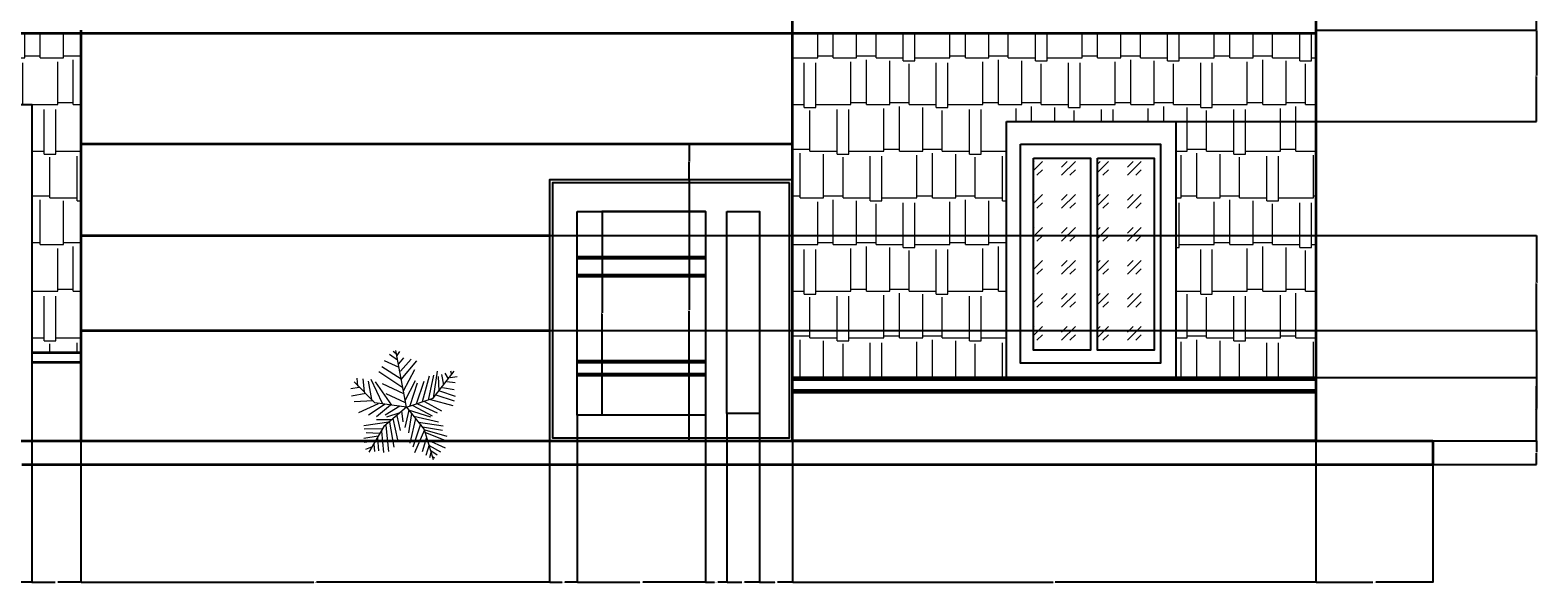
# Model space of a CAD drawing. Units: inches. Extents: x -73 to 2199, y -12 to 1583.
# Tile 2 of 3: x 686 to 2199, y -12 to 543. Entities that reach past the tile are written whole.
import ezdxf

# ---------------------------------------------------------------- set-up
doc = ezdxf.new("R2010")
doc.units = ezdxf.units.IN
doc.header["$MEASUREMENT"] = 0
for name, color, linetype, lineweight in [('A-ANNO-DIMS', 2, 'Continuous', 18), ('A-DOOR', 3, 'Continuous', 25), ('A-ELEV', 7, 'Continuous', 35), ('A-GLAZ', 4, 'Continuous', 25), ('A-GLAZ-PATT', 8, 'Continuous', 13), ('A-WALL-PATT', 8, 'Continuous', 13), ('L-PLNT', 3, 'Continuous', 18)]:
    doc.layers.add(name, color=color, linetype=linetype, lineweight=lineweight)
doc.styles.get("Standard").update_dxf_attribs({"font": 'arial.ttf'})
doc.dimstyles.get("Standard").update_dxf_attribs({"dimtxt": 0.75, "dimasz": 0.18, "dimexe": 0.18, "dimexo": 0.0625, "dimgap": 0.09, "dimtad": 0, "dimtih": 1, "dimtoh": 1, "dimdec": 4, "dimzin": 0, "dimdsep": 46, "dimlunit": 4, "dimtxsty": 'Standard', "dimcen": 0.09, "dimadec": 0, "dimazin": 0, "dimtfac": 1, "dimtdec": 4, "dimtofl": 0, "dimtmove": 0, "dimatfit": 3, "dimfxl": 1, "dimtolj": 1, "dimtzin": 0, "dimarcsym": 0})

# ---------------------------------------------------------------- blocks, each defined once
blk = doc.blocks.new('*U2')
for p, q in [((-7.288, 39.707), (-21.778, 46.673)), ((-8.737, 47.138), (-17.069, 52.711)), ((-10.186, 53.64), (-13.084, 55.962)), ((0, 0), (-10.5, 57)), ((-9.099, 51.782), (-6.563, 55.962)), ((-7.65, 43.423), (-2.578, 49.46)), ((-5.839, 35.992), (4.667, 48.067)), ((-5.114, 27.632), (10.463, 46.673)), ((-3.665, 19.273), (-27.574, 35.527)), ((-5.114, 28.097), (-24.676, 40.636)), ((-2.941, 16.486), (8.652, 37.85)), ((16.259, 5.805), (23.142, 31.348)), ((22.055, 7.198), (27.489, 32.277)), ((27, 9), (48, 36)), ((27.127, 9.056), (31.112, 35.992)), ((31.836, 30.883), (32.561, 16.486)), ((35.096, 32.741), (37.27, 22.524)), ((38.719, 34.134), (41.979, 28.561)), ((43.791, 29.954), (51.036, 30.883)), ((44.153, 36.456), (45.239, 32.741)), ((-47.498, 19.737), (-55.83, 18.344)), ((-31.5, 4.5), (-52.5, 25.5)), ((-48.585, 21.131), (-49.309, 29.026)), ((-43.513, 28.561), (-42.427, 15.558)), ((-38.442, 26.239), (-34.819, 7.663)), ((-35.544, 28.097), (-24.314, 3.947)), ((-14.533, 2.09), (-30.834, 25.31)), ((-24.314, 23.917), (-2.941, 13.7)), ((-1.129, 6.734), (9.014, 26.704)), ((3.942, 1.625), (11.187, 24.381)), ((10.101, 3.483), (17.708, 26.239)), ((33.285, 16.486), (48.862, 10.913)), ((36.183, 19.737), (48.137, 17.88)), ((40.53, 25.775), (48.862, 24.846)), ((-40.615, 13.7), (-55.105, 10.913)), ((-33.37, 6.269), (-52.207, 5.34)), ((-28.299, 3.483), (-47.86, -5.805)), ((-21.416, 3.018), (-38.079, -8.128)), ((0, 0), (-31.5, 4.5)), ((-15.982, 2.09), (-30.11, -9.521)), ((0, 0), (-22.5, -19.5)), ((-6.563, 1.161), (-21.416, -8.128)), ((-20.691, 13.7), (-1.129, 4.876)), ((0, 0), (27, 9)), ((0, 0), (18, -22.5)), ((6.478, 1.625), (26.04, -8.592)), ((11.187, 3.483), (30.749, -5.805)), ((18.07, 5.805), (35.096, -3.483)), ((24.229, 7.663), (46.688, 1.625)), ((29.662, 12.307), (48.137, 6.269)), ((-17.431, -15.094), (-42.789, -18.809)), ((-15.257, -12.772), (-30.11, -12.772)), ((-6.563, -5.805), (-19.967, -9.985)), ((-17.069, -15.094), (-12.721, -40.172)), ((-13.446, -11.378), (-8.737, -32.741)), ((-9.461, -8.592), (-6.201, -23.453)), ((-4.752, -3.483), (-3.665, -14.629)), ((2.493, -3.019), (-1.491, -20.202)), ((1.769, -2.555), (24.229, -9.521)), ((5.029, -6.27), (2.131, -25.775)), ((9.014, -11.378), (3.58, -35.992)), ((7.565, -9.056), (32.198, -14.629)), ((12.274, -15.094), (36.907, -18.809)), ((-28.299, -29.026), (-42.789, -31.348)), ((-24.314, -21.596), (-42.427, -22.06)), ((-26.849, -26.24), (-40.253, -25.775)), ((-22.5, -19.5), (-37.5, -45)), ((-25.038, -23.918), (-22.865, -45.281)), ((-20.691, -18.345), (-17.793, -44.352)), ((14.085, -16.951), (6.478, -40.172)), ((18.07, -22.524), (8.289, -45.745)), ((16.259, -19.738), (36.183, -22.989)), ((18, -22.5), (27, -52.5)), ((18.433, -22.524), (40.53, -29.026)), ((19.157, -25.311), (38.719, -33.206)), ((-30.834, -34.135), (-42.427, -35.528)), ((-34.457, -39.708), (-40.978, -42.494)), ((-32.646, -36.921), (-31.921, -44.352)), ((-29.023, -30.884), (-27.936, -43.887)), ((20.244, -30.419), (15.897, -44.816)), ((22.78, -37.85), (19.519, -48.532)), ((21.331, -32.741), (39.081, -40.636)), ((22.78, -38.314), (34.372, -44.816)), ((24.591, -43.423), (30.749, -47.603)), ((24.591, -45.745), (23.142, -50.854)), ((26.764, -49.925), (28.213, -50.854))]:
    blk.add_line(p, q)
blk = doc.blocks.new('WIN-GLAZED-TALL')
for points in [[(1665.6, 878.6), (1835.3, 878.6), (1835.3, 622.1), (1665.6, 622.1)], [(1679.7, 855.9), (1819.9, 855.9), (1819.9, 636.5), (1679.7, 636.5)], [(1692.7, 842.1), (1749.8, 842.1), (1749.8, 649.4), (1692.7, 649.4)], [(1756.7, 842.1), (1813.8, 842.1), (1813.8, 649.4), (1756.7, 649.4)]]:
    blk.add_lwpolyline(points, close=True)
blk = doc.blocks.new('*D16')
at = {"layer": 'A-ANNO-DIMS', "color": 0, "lineweight": -2, "transparency": 16777216}
for p, q in [((87.8, 130.9), (87.8, -11.2)), ((687.8, 130.9), (687.8, -11.2)), ((88, -11), (386.4, -11)), ((687.6, -11), (389.2, -11))]:
    blk.add_line(p, q, dxfattribs=at)
at = {"layer": 'A-ANNO-DIMS', "color": 0, "transparency": 16777216}
for points in [[(88, -11), (88, -11.1), (87.8, -11)], [(687.6, -11), (687.6, -11.1), (687.8, -11)]]:
    blk.add_solid(points, dxfattribs=at)
at = {"layer": 'Defpoints', "color": 0, "transparency": 16777216}
for p in [(87.8, 131), (687.8, 131), (687.8, -11)]:
    blk.add_point(p, dxfattribs=at)
at = {"layer": 'A-ANNO-DIMS', "color": 0, "transparency": 16777216, "insert": (387.8, -11), "char_height": 0.75, "attachment_point": 5}
blk.add_mtext('\\A1;599.9', dxfattribs=at)
blk = doc.blocks.new('*D17')
at = {"layer": 'A-ANNO-DIMS', "color": 0, "lineweight": -2, "transparency": 16777216}
for p, q in [((687.8, 130.9), (687.8, -11.2)), ((736.9, 130.9), (736.9, -11.2)), ((687.9, -11), (711, -11)), ((736.7, -11), (713.7, -11))]:
    blk.add_line(p, q, dxfattribs=at)
at = {"layer": 'A-ANNO-DIMS', "color": 0, "transparency": 16777216}
for points in [[(687.9, -11), (687.9, -11.1), (687.8, -11)], [(736.7, -11), (736.7, -11.1), (736.9, -11)]]:
    blk.add_solid(points, dxfattribs=at)
at = {"layer": 'Defpoints', "color": 0, "transparency": 16777216}
for p in [(687.8, 131), (736.9, 131), (736.9, -11)]:
    blk.add_point(p, dxfattribs=at)
at = {"layer": 'A-ANNO-DIMS', "color": 0, "transparency": 16777216, "insert": (712.3, -11), "char_height": 0.75, "attachment_point": 5}
blk.add_mtext('\\A1;49.14', dxfattribs=at)
blk = doc.blocks.new('*D18')
at = {"layer": 'A-ANNO-DIMS', "color": 0, "lineweight": -2, "transparency": 16777216}
for p, q in [((736.9, 130.9), (736.9, -11.2)), ((1207.2, 130.9), (1207.2, -11.2)), ((737.1, -11), (970.7, -11)), ((1207, -11), (973.4, -11))]:
    blk.add_line(p, q, dxfattribs=at)
at = {"layer": 'A-ANNO-DIMS', "color": 0, "transparency": 16777216}
for points in [[(737.1, -11), (737.1, -11.1), (736.9, -11)], [(1207, -11), (1207, -11.1), (1207.2, -11)]]:
    blk.add_solid(points, dxfattribs=at)
at = {"layer": 'Defpoints', "color": 0, "transparency": 16777216}
for p in [(736.9, 131), (1207.2, 131), (1207.2, -11)]:
    blk.add_point(p, dxfattribs=at)
at = {"layer": 'A-ANNO-DIMS', "color": 0, "transparency": 16777216, "insert": (972, -11), "char_height": 0.75, "attachment_point": 5}
blk.add_mtext('\\A1;470.3', dxfattribs=at)
blk = doc.blocks.new('*D19')
at = {"layer": 'A-ANNO-DIMS', "color": 0, "lineweight": -2, "transparency": 16777216}
for p, q in [((1234.9, 156.6), (1234.9, -11.2)), ((1207.2, 130.9), (1207.2, -11.2)), ((1207.3, -11), (1219.7, -11)), ((1234.7, -11), (1222.4, -11))]:
    blk.add_line(p, q, dxfattribs=at)
at = {"layer": 'A-ANNO-DIMS', "color": 0, "transparency": 16777216}
for points in [[(1207.3, -11), (1207.3, -11.1), (1207.2, -11)], [(1234.7, -11), (1234.7, -11.1), (1234.9, -11)]]:
    blk.add_solid(points, dxfattribs=at)
at = {"layer": 'Defpoints', "color": 0, "transparency": 16777216}
for p in [(1234.9, 156.6), (1207.2, 131), (1234.9, -11)]:
    blk.add_point(p, dxfattribs=at)
at = {"layer": 'A-ANNO-DIMS', "color": 0, "transparency": 16777216, "insert": (1221, -11), "char_height": 0.75, "attachment_point": 5}
blk.add_mtext('\\A1;27.73', dxfattribs=at)
blk = doc.blocks.new('*D20')
at = {"layer": 'A-ANNO-DIMS', "color": 0, "lineweight": -2, "transparency": 16777216}
for p, q in [((1234.9, 156.6), (1234.9, -11.2)), ((1363.6, 156.6), (1363.6, -11.2)), ((1235.1, -11), (1297.6, -11)), ((1363.4, -11), (1300.8, -11))]:
    blk.add_line(p, q, dxfattribs=at)
at = {"layer": 'A-ANNO-DIMS', "color": 0, "transparency": 16777216}
for points in [[(1235.1, -11), (1235.1, -11.1), (1234.9, -11)], [(1363.4, -11), (1363.4, -11.1), (1363.6, -11)]]:
    blk.add_solid(points, dxfattribs=at)
at = {"layer": 'Defpoints', "color": 0, "transparency": 16777216}
for p in [(1234.9, 156.6), (1363.6, 156.6), (1363.6, -11)]:
    blk.add_point(p, dxfattribs=at)
at = {"layer": 'A-ANNO-DIMS', "color": 0, "transparency": 16777216, "insert": (1299.2, -11), "char_height": 0.75, "attachment_point": 5}
blk.add_mtext('\\A1;128.67', dxfattribs=at)
blk = doc.blocks.new('*D21')
at = {"layer": 'A-ANNO-DIMS', "color": 0, "lineweight": -2, "transparency": 16777216}
for p, q in [((1363.6, 156.6), (1363.6, -11.2)), ((1385.1, 158.2), (1385.1, -11.2)), ((1363.7, -11), (1372.7, -11)), ((1384.9, -11), (1376, -11))]:
    blk.add_line(p, q, dxfattribs=at)
at = {"layer": 'A-ANNO-DIMS', "color": 0, "transparency": 16777216}
for points in [[(1363.7, -11), (1363.7, -11.1), (1363.6, -11)], [(1384.9, -11), (1384.9, -11.1), (1385.1, -11)]]:
    blk.add_solid(points, dxfattribs=at)
at = {"layer": 'Defpoints', "color": 0, "transparency": 16777216}
for p in [(1363.6, 156.6), (1385.1, 158.3), (1385.1, -11)]:
    blk.add_point(p, dxfattribs=at)
at = {"layer": 'A-ANNO-DIMS', "color": 0, "transparency": 16777216, "insert": (1374.3, -11), "char_height": 0.75, "attachment_point": 5}
blk.add_mtext('\\A1;21.538', dxfattribs=at)
blk = doc.blocks.new('*D22')
at = {"layer": 'A-ANNO-DIMS', "color": 0, "lineweight": -2, "transparency": 16777216}
for p, q in [((1385.1, 158.2), (1385.1, -11.2)), ((1417.7, 158.2), (1417.7, -11.2)), ((1385.3, -11), (1400, -11)), ((1417.5, -11), (1402.8, -11))]:
    blk.add_line(p, q, dxfattribs=at)
at = {"layer": 'A-ANNO-DIMS', "color": 0, "transparency": 16777216}
for points in [[(1385.3, -11), (1385.3, -11.1), (1385.1, -11)], [(1417.5, -11), (1417.5, -11.1), (1417.7, -11)]]:
    blk.add_solid(points, dxfattribs=at)
at = {"layer": 'Defpoints', "color": 0, "transparency": 16777216}
for p in [(1385.1, 158.3), (1417.7, 158.3), (1417.7, -11)]:
    blk.add_point(p, dxfattribs=at)
at = {"layer": 'A-ANNO-DIMS', "color": 0, "transparency": 16777216, "insert": (1401.4, -11), "char_height": 0.75, "attachment_point": 5}
blk.add_mtext('\\A1;32.58', dxfattribs=at)
blk = doc.blocks.new('*D23')
at = {"layer": 'A-ANNO-DIMS', "color": 0, "lineweight": -2, "transparency": 16777216}
for p, q in [((1417.7, 158.2), (1417.7, -11.2)), ((1451, 130.9), (1451, -11.2)), ((1417.9, -11), (1433, -11)), ((1450.8, -11), (1435.7, -11))]:
    blk.add_line(p, q, dxfattribs=at)
at = {"layer": 'A-ANNO-DIMS', "color": 0, "transparency": 16777216}
for points in [[(1417.9, -11), (1417.9, -11.1), (1417.7, -11)], [(1450.8, -11), (1450.8, -11.1), (1451, -11)]]:
    blk.add_solid(points, dxfattribs=at)
at = {"layer": 'Defpoints', "color": 0, "transparency": 16777216}
for p in [(1417.7, 158.3), (1451, 131), (1451, -11)]:
    blk.add_point(p, dxfattribs=at)
at = {"layer": 'A-ANNO-DIMS', "color": 0, "transparency": 16777216, "insert": (1434.3, -11), "char_height": 0.75, "attachment_point": 5}
blk.add_mtext('\\A1;33.27', dxfattribs=at)
blk = doc.blocks.new('*D24')
at = {"layer": 'A-ANNO-DIMS', "color": 0, "lineweight": -2, "transparency": 16777216}
for p, q in [((1451, 130.9), (1451, -11.2)), ((1976, 130.9), (1976, -11.2)), ((1451.1, -11), (1712.5, -11)), ((1975.8, -11), (1714.4, -11))]:
    blk.add_line(p, q, dxfattribs=at)
at = {"layer": 'A-ANNO-DIMS', "color": 0, "transparency": 16777216}
for points in [[(1451.1, -11), (1451.1, -11.1), (1451, -11)], [(1975.8, -11), (1975.8, -11.1), (1976, -11)]]:
    blk.add_solid(points, dxfattribs=at)
at = {"layer": 'Defpoints', "color": 0, "transparency": 16777216}
for p in [(1451, 131), (1976, 131), (1976, -11)]:
    blk.add_point(p, dxfattribs=at)
at = {"layer": 'A-ANNO-DIMS', "color": 0, "transparency": 16777216, "insert": (1713.5, -11), "char_height": 0.75, "attachment_point": 5}
blk.add_mtext('\\A1;525', dxfattribs=at)
blk = doc.blocks.new('*D25')
at = {"layer": 'A-ANNO-DIMS', "color": 0, "lineweight": -2, "transparency": 16777216}
for p, q in [((1976, 130.9), (1976, -11.2)), ((2093.3, 130.9), (2093.3, -11.2)), ((1976.1, -11), (2033, -11)), ((2093.1, -11), (2036.2, -11))]:
    blk.add_line(p, q, dxfattribs=at)
at = {"layer": 'A-ANNO-DIMS', "color": 0, "transparency": 16777216}
for points in [[(1976.1, -11), (1976.1, -11.1), (1976, -11)], [(2093.1, -11), (2093.1, -11.1), (2093.3, -11)]]:
    blk.add_solid(points, dxfattribs=at)
at = {"layer": 'Defpoints', "color": 0, "transparency": 16777216}
for p in [(1976, 131), (2093.3, 131), (2093.3, -11)]:
    blk.add_point(p, dxfattribs=at)
at = {"layer": 'A-ANNO-DIMS', "color": 0, "transparency": 16777216, "insert": (2034.6, -11), "char_height": 0.75, "attachment_point": 5}
blk.add_mtext('\\A1;117.34', dxfattribs=at)
blk = doc.blocks.new('*D41')
at = {"layer": 'A-ANNO-DIMS', "color": 0, "lineweight": -2, "transparency": 16777216}
for p, q in [((2093.4, 131), (2197.2, 131)), ((2197.1, 130.8), (2197.1, 119.5)), ((2093.4, 107), (2197.2, 107)), ((2197.1, 107.2), (2197.1, 118.5))]:
    blk.add_line(p, q, dxfattribs=at)
at = {"layer": 'A-ANNO-DIMS', "color": 0, "transparency": 16777216}
for points in [[(2197, 130.8), (2197.1, 130.8), (2197.1, 131)], [(2197, 107.2), (2197.1, 107.2), (2197.1, 107)]]:
    blk.add_solid(points, dxfattribs=at)
at = {"layer": 'Defpoints', "color": 0, "transparency": 16777216}
for p in [(2093.3, 131), (2197.1, 131), (2093.3, 107)]:
    blk.add_point(p, dxfattribs=at)
at = {"layer": 'A-ANNO-DIMS', "color": 0, "transparency": 16777216, "insert": (2197.1, 119), "char_height": 0.75, "attachment_point": 5}
blk.add_mtext('\\A1;24', dxfattribs=at)
blk = doc.blocks.new('*D42')
at = {"layer": 'A-ANNO-DIMS', "color": 0, "lineweight": -2, "transparency": 16777216}
for p, q in [((1835.4, 194.5), (2197.2, 194.5)), ((2197.1, 194.3), (2197.1, 163.2)), ((2197.1, 131.2), (2197.1, 162.3)), ((1976, 131), (2197.2, 131))]:
    blk.add_line(p, q, dxfattribs=at)
at = {"layer": 'A-ANNO-DIMS', "color": 0, "transparency": 16777216}
for points in [[(2197, 194.3), (2197.1, 194.3), (2197.1, 194.5)], [(2197, 131.2), (2197.1, 131.2), (2197.1, 131)]]:
    blk.add_solid(points, dxfattribs=at)
at = {"layer": 'Defpoints', "color": 0, "transparency": 16777216}
for p in [(1835.3, 194.5), (2197.1, 194.5), (1976, 131)]:
    blk.add_point(p, dxfattribs=at)
at = {"layer": 'A-ANNO-DIMS', "color": 0, "transparency": 16777216, "insert": (2197.1, 162.7), "char_height": 0.75, "attachment_point": 5}
blk.add_mtext('\\A1;63.45', dxfattribs=at)
blk = doc.blocks.new('*D43')
at = {"layer": 'A-ANNO-DIMS', "color": 0, "lineweight": -2, "transparency": 16777216}
for p, q in [((1976, 542.7), (2197.2, 542.7)), ((2197.1, 542.5), (2197.1, 497.3)), ((2197.1, 451.1), (2197.1, 496.4)), ((1835.4, 451), (2197.2, 451))]:
    blk.add_line(p, q, dxfattribs=at)
at = {"layer": 'A-ANNO-DIMS', "color": 0, "transparency": 16777216}
for points in [[(2197, 542.5), (2197.1, 542.5), (2197.1, 542.7)], [(2197, 451.1), (2197.1, 451.1), (2197.1, 451)]]:
    blk.add_solid(points, dxfattribs=at)
at = {"layer": 'Defpoints', "color": 0, "transparency": 16777216}
for p in [(1976, 542.7), (2197.1, 542.7), (1835.3, 451)]:
    blk.add_point(p, dxfattribs=at)
at = {"layer": 'A-ANNO-DIMS', "color": 0, "transparency": 16777216, "insert": (2197.1, 496.8), "char_height": 0.75, "attachment_point": 5}
blk.add_mtext('\\A1;91.74', dxfattribs=at)
blk = doc.blocks.new('*D44')
at = {"layer": 'A-ANNO-DIMS', "color": 0, "lineweight": -2, "transparency": 16777216}
for p, q in [((1835.4, 622.1), (2197.2, 622.1)), ((2197.1, 621.9), (2197.1, 582.9)), ((2197.1, 542.9), (2197.1, 581.9)), ((1976, 542.7), (2197.2, 542.7))]:
    blk.add_line(p, q, dxfattribs=at)
at = {"layer": 'A-ANNO-DIMS', "color": 0, "transparency": 16777216}
for points in [[(2197, 621.9), (2197.1, 621.9), (2197.1, 622.1)], [(2197, 542.9), (2197.1, 542.9), (2197.1, 542.7)]]:
    blk.add_solid(points, dxfattribs=at)
at = {"layer": 'Defpoints', "color": 0, "transparency": 16777216}
for p in [(1835.3, 622.1), (2197.1, 622.1), (1976, 542.7)]:
    blk.add_point(p, dxfattribs=at)
at = {"layer": 'A-ANNO-DIMS', "color": 0, "transparency": 16777216, "insert": (2197.1, 582.4), "char_height": 0.75, "attachment_point": 5}
blk.add_mtext('\\A1;79.39', dxfattribs=at)
blk = doc.blocks.new('*D53')
at = {"layer": 'A-ANNO-DIMS', "color": 0, "lineweight": -2, "transparency": 16777216}
for p, q in [((1363.5, 360.8), (1259.6, 360.8)), ((1259.8, 360.6), (1259.8, 259.2)), ((1259.8, 156.8), (1259.8, 258.2)), ((1363.5, 156.6), (1259.6, 156.6))]:
    blk.add_line(p, q, dxfattribs=at)
at = {"layer": 'A-ANNO-DIMS', "color": 0, "transparency": 16777216}
for points in [[(1259.8, 360.6), (1259.8, 360.6), (1259.8, 360.8)], [(1259.8, 156.8), (1259.8, 156.8), (1259.8, 156.6)]]:
    blk.add_solid(points, dxfattribs=at)
at = {"layer": 'Defpoints', "color": 0, "transparency": 16777216}
for p in [(1259.8, 360.8), (1363.6, 360.8), (1363.6, 156.6)]:
    blk.add_point(p, dxfattribs=at)
at = {"layer": 'A-ANNO-DIMS', "color": 0, "transparency": 16777216, "insert": (1259.8, 258.7), "char_height": 0.75, "attachment_point": 5}
blk.add_mtext('\\A1;204.17', dxfattribs=at)
blk = doc.blocks.new('*D54')
at = {"layer": 'A-ANNO-DIMS', "color": 0, "lineweight": -2, "transparency": 16777216}
for p, q in [((1450.9, 392.5), (1347, 392.5)), ((1347.2, 392.4), (1347.2, 262.2)), ((1347.2, 131.2), (1347.2, 261.3)), ((1450.9, 131), (1347, 131))]:
    blk.add_line(p, q, dxfattribs=at)
at = {"layer": 'A-ANNO-DIMS', "color": 0, "transparency": 16777216}
for points in [[(1347.2, 392.4), (1347.2, 392.4), (1347.2, 392.5)], [(1347.2, 131.2), (1347.2, 131.2), (1347.2, 131)]]:
    blk.add_solid(points, dxfattribs=at)
at = {"layer": 'Defpoints', "color": 0, "transparency": 16777216}
for p in [(1347.2, 392.5), (1451, 392.5), (1451, 131)]:
    blk.add_point(p, dxfattribs=at)
at = {"layer": 'A-ANNO-DIMS', "color": 0, "transparency": 16777216, "insert": (1347.2, 261.8), "char_height": 0.75, "attachment_point": 5}
blk.add_mtext('\\A1;261.53', dxfattribs=at)
blk = doc.blocks.new('*D55')
at = {"layer": 'A-ANNO-DIMS', "color": 0, "lineweight": -2, "transparency": 16777216}
for p, q in [((1207.2, 241.6), (2197.2, 241.6)), ((2197.1, 241.4), (2197.1, 186.8)), ((2197.1, 131.2), (2197.1, 185.8)), ((1207.2, 131), (2197.2, 131))]:
    blk.add_line(p, q, dxfattribs=at)
at = {"layer": 'A-ANNO-DIMS', "color": 0, "transparency": 16777216}
for points in [[(2197, 241.4), (2197.1, 241.4), (2197.1, 241.6)], [(2197, 131.2), (2197.1, 131.2), (2197.1, 131)]]:
    blk.add_solid(points, dxfattribs=at)
at = {"layer": 'Defpoints', "color": 0, "transparency": 16777216}
for p in [(1207.2, 241.6), (2197.1, 241.6), (1207.2, 131)]:
    blk.add_point(p, dxfattribs=at)
at = {"layer": 'A-ANNO-DIMS', "color": 0, "transparency": 16777216, "insert": (2197.1, 186.3), "char_height": 0.75, "attachment_point": 5}
blk.add_mtext('\\A1;110.56', dxfattribs=at)
blk = doc.blocks.new('*D56')
at = {"layer": 'A-ANNO-DIMS', "color": 0, "lineweight": -2, "transparency": 16777216}
for p, q in [((1207.2, 336.9), (2197.2, 336.9)), ((2197.1, 336.7), (2197.1, 289.7)), ((2197.1, 241.8), (2197.1, 288.7)), ((1207.2, 241.6), (2197.2, 241.6))]:
    blk.add_line(p, q, dxfattribs=at)
at = {"layer": 'A-ANNO-DIMS', "color": 0, "transparency": 16777216}
for points in [[(2197, 336.7), (2197.1, 336.7), (2197.1, 336.9)], [(2197, 241.8), (2197.1, 241.8), (2197.1, 241.6)]]:
    blk.add_solid(points, dxfattribs=at)
at = {"layer": 'Defpoints', "color": 0, "transparency": 16777216}
for p in [(1207.2, 336.9), (2197.1, 336.9), (1207.2, 241.6)]:
    blk.add_point(p, dxfattribs=at)
at = {"layer": 'A-ANNO-DIMS', "color": 0, "transparency": 16777216, "insert": (2197.1, 289.2), "char_height": 0.75, "attachment_point": 5}
blk.add_mtext('\\A1;95.29', dxfattribs=at)
blk = doc.blocks.new('*D57')
at = {"layer": 'A-ANNO-DIMS', "color": 0, "lineweight": -2, "transparency": 16777216}
for p, q in [((1450.9, 428.7), (1347, 428.7)), ((1347.2, 428.5), (1347.2, 411.1)), ((1347.2, 392.7), (1347.2, 410.2)), ((1450.9, 392.5), (1347, 392.5))]:
    blk.add_line(p, q, dxfattribs=at)
at = {"layer": 'A-ANNO-DIMS', "color": 0, "transparency": 16777216}
for points in [[(1347.2, 428.5), (1347.2, 428.5), (1347.2, 428.7)], [(1347.2, 392.7), (1347.2, 392.7), (1347.2, 392.5)]]:
    blk.add_solid(points, dxfattribs=at)
at = {"layer": 'Defpoints', "color": 0, "transparency": 16777216}
for p in [(1347.2, 428.7), (1451, 428.7), (1451, 392.5)]:
    blk.add_point(p, dxfattribs=at)
at = {"layer": 'A-ANNO-DIMS', "color": 0, "transparency": 16777216, "insert": (1347.2, 410.6), "char_height": 0.75, "attachment_point": 5}
blk.add_mtext('\\A1;36.17', dxfattribs=at)

msp = doc.modelspace()

# ---------------------------------------------------------------- hatches: boundary and pattern name
at = {"layer": 'A-GLAZ-PATT'}
h = msp.add_hatch(dxfattribs=at)
h.set_pattern_fill('GOST_GLASS', color=256, scale=3.9)
h.set_pattern_definition([(45, (0, 0), (33.0926, 0), [19.5, -27.3]), (45, (8.273, 0), (33.0926, 0), [7.8, -39]), (45, (0, 8.273), (33.0926, 0), [7.8, -39])])
h.paths.add_polyline_path([(1813.8199, 842.1341), (1756.6853, 842.1341), (1756.6853, 649.4087), (1813.8199, 649.4087)])
h.paths.add_polyline_path([(1749.7931, 842.1341), (1692.6585, 842.1341), (1692.6585, 649.4087), (1749.7931, 649.4087)])
h.paths.add_polyline_path([(1813.8199, 414.5003), (1756.6853, 414.5003), (1756.6853, 221.7748), (1813.8199, 221.7748)])
h.paths.add_polyline_path([(1749.7931, 414.5003), (1692.6585, 414.5003), (1692.6585, 221.7748), (1749.7931, 221.7748)])
at = {"layer": 'A-WALL-PATT'}
h = msp.add_hatch(dxfattribs=at)
h.set_pattern_fill('AR-RSHKE', color=256, scale=3.9)
h.paths.add_polyline_path([(736.9068, 539.7065), (42.6128, 539.7065), (42.6128, 419.0114), (42.6128, 219.3768), (87.8284, 219.3768), (87.8284, 468.215), (687.7643, 468.215), (687.7643, 219.3768), (736.9068, 219.3768)])
h.paths.add_polyline_path([(1665.5962, 450.9629), (1835.312, 450.9629), (1835.312, 194.4603), (1975.9662, 194.4603), (1975.9662, 539.7065), (1450.9568, 539.7065), (1450.9568, 194.4603), (1665.5962, 194.4603)])

# ---------------------------------------------------------------- linework, layer by layer
at = {"layer": 'A-DOOR'}
for p, q in [((1234.8955, 315.7313), (1363.5695, 315.7313)), ((1234.8955, 313.7313), (1363.5695, 313.7313)), ((1234.8955, 297.6756), (1363.5695, 297.6756)), ((1234.8955, 295.6756), (1363.5695, 295.6756)), ((1234.8955, 211.543), (1363.5695, 211.543)), ((1234.8955, 209.543), (1363.5695, 209.543)), ((1234.8955, 198.3899), (1363.5695, 198.3899)), ((1234.8955, 196.3899), (1363.5695, 196.3899))]:
    msp.add_line(p, q, dxfattribs=at)
for points in [[(87.8284, 468.215), (687.7643, 468.215), (687.7643, 131.0114), (87.8284, 131.0114)], [(1450.9568, 392.5409), (1207.1659, 392.5409), (1207.1659, 131.0114), (1450.9568, 131.0114)], [(1447.9568, 389.5409), (1210.1659, 389.5409), (1210.1659, 134.0114), (1447.9568, 134.0114)], [(1234.8955, 360.7973), (1363.5695, 360.7973), (1363.5695, 156.6289), (1234.8955, 156.6289)], [(1385.1072, 360.7973), (1417.6899, 360.7973), (1417.6899, 158.2843), (1385.1072, 158.2843)]]:
    msp.add_lwpolyline(points, close=True, dxfattribs=at)
at = {"layer": 'A-ELEV'}
for p, q in [((42.6128, 539.7065), (736.9068, 539.7065)), ((736.9068, 542.7065), (736.9068, 131.0114)), ((736.9068, 539.7065), (1975.9662, 539.7065)), ((736.9068, 428.7143), (1450.9568, 428.7143)), ((736.9068, 336.8589), (1207.1659, 336.8589)), ((736.9068, 241.5726), (1207.1659, 241.5726)), ((687.7643, 219.3768), (736.9068, 219.3768)), ((687.7643, 209.5972), (736.9068, 209.5972)), ((691.6912, 209.5972), (736.9068, 209.5972)), ((1450.9568, 194.4603), (1975.9662, 194.4603)), ((1450.9568, 192.4603), (1975.9662, 192.4603)), ((1450.9568, 181.7048), (1975.9662, 181.7048)), ((1450.9568, 179.7048), (1975.9662, 179.7048)), ((675.9771, 131.0114), (1134.5569, 131.0114)), ((1134.5569, 131.0114), (2093.3026, 131.0114)), ((2093.3026, 131.0114), (2093.3026, 107.0114)), ((677.7181, 107.0114), (1212.2414, 107.0114)), ((1212.2414, 107.0114), (2093.3026, 107.0114))]:
    msp.add_line(p, q, dxfattribs=at)
msp.add_lwpolyline([(1450.9568, 1020.5741), (1975.9662, 1020.5741), (1975.9662, 131.0114), (1450.9568, 131.0114)], close=True, dxfattribs=at)

# ---------------------------------------------------------------- block references
at = {"layer": 'A-GLAZ'}
msp.add_blockref('WIN-GLAZED-TALL', (0, -427.6339), dxfattribs=at)
at = {"layer": 'L-PLNT'}
msp.add_blockref('*U2', (1063.4721, 164.5874), dxfattribs=at)

# ---------------------------------------------------------------- dimensions: what is measured, and where the dimension line sits
at = {"layer": 'A-ANNO-DIMS'}
for base, p1, p2, override, picture, middle in [((2197.0526, 622.0942), (1975.9662, 542.7065), (1835.312, 622.0942), {"dimdec": 2, "dimlfac": 1, "dimrnd": 0, "dimzin": 0, "dimdsep": 46, "dimlunit": 2}, '*D44', (2197.0526, 582.4004)), ((2197.0526, 542.7065), (1835.312, 450.9629), (1975.9662, 542.7065), {"dimdec": 2, "dimlfac": 1, "dimrnd": 0, "dimzin": 0, "dimdsep": 46, "dimlunit": 2}, '*D43', (2197.0526, 496.8347)), ((1347.2068, 428.7143), (1450.9568, 392.5409), (1450.9568, 428.7143), {"dimdec": 2, "dimlfac": 1, "dimrnd": 0, "dimzin": 0, "dimdsep": 46, "dimlunit": 2}, '*D57', (1347.2068, 410.6276)), ((1347.2068, 392.5409), (1450.9568, 131.0114), (1450.9568, 392.5409), {"dimdec": 2, "dimlfac": 1, "dimrnd": 0, "dimzin": 0, "dimdsep": 46, "dimlunit": 2}, '*D54', (1347.2068, 261.7762)), ((1259.8195, 360.7973), (1363.5695, 156.6289), (1363.5695, 360.7973), {"dimdec": 2, "dimlfac": 1, "dimrnd": 0, "dimzin": 0, "dimdsep": 46, "dimlunit": 2}, '*D53', (1259.8195, 258.7131)), ((2197.0526, 336.8589), (1207.1659, 241.5726), (1207.1659, 336.8589), {"dimdec": 2, "dimlfac": 1, "dimrnd": 0, "dimzin": 0, "dimdsep": 46, "dimlunit": 2}, '*D56', (2197.0526, 289.2158)), ((2197.0526, 241.5726), (1207.1659, 131.0114), (1207.1659, 241.5726), {"dimdec": 2, "dimlfac": 1, "dimrnd": 0, "dimzin": 0, "dimdsep": 46, "dimlunit": 2}, '*D55', (2197.0526, 186.292)), ((2197.0526, 194.4603), (1975.9662, 131.0114), (1835.312, 194.4603), {"dimdec": 2, "dimlfac": 1, "dimrnd": 0, "dimzin": 0, "dimdsep": 46, "dimlunit": 2}, '*D42', (2197.0526, 162.7358)), ((2197.0526, 131.0114), (2093.3026, 107.0114), (2093.3026, 131.0114), {"dimdec": 0, "dimlfac": 1, "dimrnd": 0, "dimzin": 0, "dimdsep": 46, "dimlunit": 2}, '*D41', (2197.0526, 119.0114))]:
    dim = msp.add_linear_dim(base=base, p1=p1, p2=p2, angle=90, dimstyle='Standard', override=override, dxfattribs=at)
    dim.commit()
    dim.dimension.update_dxf_attribs({"geometry": picture, "text_midpoint": middle})
for base, p1, p2, override, picture, middle in [((1234.8955, -11.0496), (1207.1659, 131.0114), (1234.8955, 156.6289), {"dimdec": 2, "dimlfac": 1, "dimrnd": 0, "dimzin": 0, "dimdsep": 46, "dimlunit": 2}, '*D19', (1221.0307, -11.0496)), ((1363.5695, -11.0496), (1234.8955, 156.6289), (1363.5695, 156.6289), {"dimdec": 2, "dimlfac": 1, "dimrnd": 0, "dimzin": 0, "dimdsep": 46, "dimlunit": 2}, '*D20', (1299.2325, -11.0496)), ((1385.1072, -11.0496), (1363.5695, 156.6289), (1385.1072, 158.2843), {"dimdec": 3, "dimlfac": 1, "dimrnd": 0, "dimzin": 0, "dimdsep": 46, "dimlunit": 2}, '*D21', (1374.3384, -11.0496)), ((1417.6899, -11.0496), (1385.1072, 158.2843), (1417.6899, 158.2843), {"dimdec": 2, "dimlfac": 1, "dimrnd": 0, "dimzin": 0, "dimdsep": 46, "dimlunit": 2}, '*D22', (1401.3985, -11.0496)), ((1450.9568, -11.0496), (1417.6899, 158.2843), (1450.9568, 131.0114), {"dimdec": 2, "dimlfac": 1, "dimrnd": 0, "dimzin": 0, "dimdsep": 46, "dimlunit": 2}, '*D23', (1434.3233, -11.0496)), ((687.7643, -11.0496), (87.8284, 131.0114), (687.7643, 131.0114), {"dimdec": 1, "dimlfac": 1, "dimrnd": 0, "dimzin": 0, "dimdsep": 46, "dimlunit": 2}, '*D16', (387.7963, -11.0496)), ((736.9068, -11.0496), (687.7643, 131.0114), (736.9068, 131.0114), {"dimdec": 2, "dimlfac": 1, "dimrnd": 0, "dimzin": 0, "dimdsep": 46, "dimlunit": 2}, '*D17', (712.3355, -11.0496)), ((1207.1659, -11.0496), (736.9068, 131.0114), (1207.1659, 131.0114), {"dimdec": 1, "dimlfac": 1, "dimrnd": 0, "dimzin": 0, "dimdsep": 46, "dimlunit": 2}, '*D18', (972.0364, -11.0496)), ((1975.9662, -11.0496), (1450.9568, 131.0114), (1975.9662, 131.0114), {"dimdec": 0, "dimlfac": 1, "dimrnd": 0, "dimzin": 0, "dimdsep": 46, "dimlunit": 2}, '*D24', (1713.4615, -11.0496)), ((2093.3026, -11.0496), (1975.9662, 131.0114), (2093.3026, 131.0114), {"dimdec": 2, "dimlfac": 1, "dimrnd": 0, "dimzin": 0, "dimdsep": 46, "dimlunit": 2}, '*D25', (2034.6344, -11.0496))]:
    dim = msp.add_linear_dim(base=base, p1=p1, p2=p2, dimstyle='Standard', override=override, dxfattribs=at)
    dim.commit()
    dim.dimension.update_dxf_attribs({"geometry": picture, "text_midpoint": middle})

doc.saveas('drawing.dxf')
